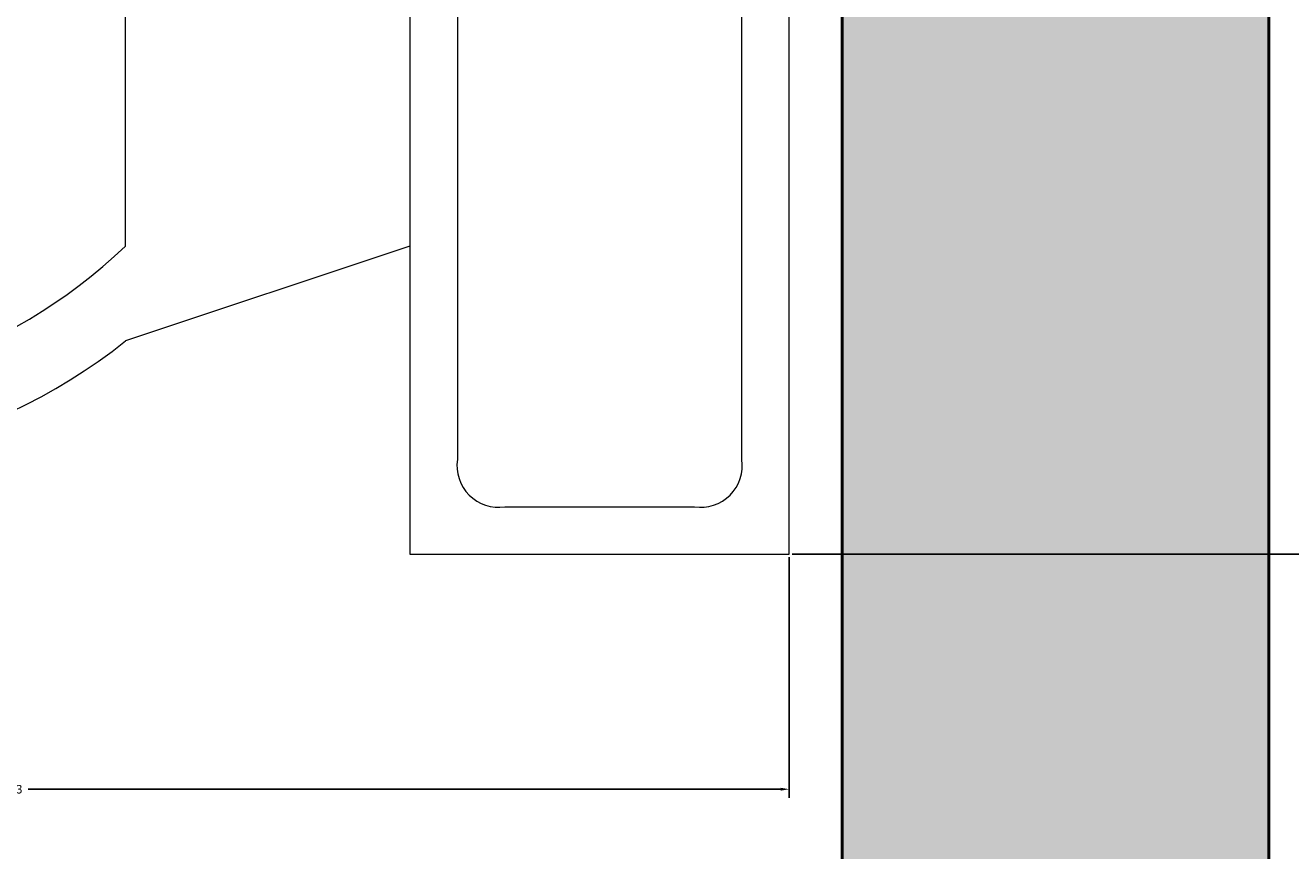
# Model space of a CAD drawing. Units: inches. Extents: x 2307 to 2544, y 2171 to 2540.
# Tile 49 of 52: x 2498 to 2525, y 2482 to 2499. Entities that reach past the tile are written whole.
import ezdxf

# ---------------------------------------------------------------- set-up
doc = ezdxf.new("R2010")
doc.units = ezdxf.units.IN
for name, color, linetype, lineweight in [('A-ANNO-DIMS', 2, 'Continuous', 18), ('A-FLOR-FIXT', 9, 'Continuous', 18), ('A-WALL', 7, 'Continuous', 50)]:
    doc.layers.add(name, color=color, linetype=linetype, lineweight=lineweight)
doc.layers.add('A-WALL-PATT', color=18, linetype='Continuous', lineweight=13, true_color=0x000000)
doc.styles.get("Standard").update_dxf_attribs({"font": 'arial.ttf'})
doc.dimstyles.get("Standard").update_dxf_attribs({"dimtxt": 0.18, "dimasz": 0.18, "dimexe": 0.18, "dimexo": 0.0625, "dimgap": 0.09, "dimtad": 0, "dimtih": 1, "dimtoh": 1, "dimdec": 4, "dimzin": 0, "dimdsep": 46, "dimtxsty": 'Standard', "dimcen": 0.09, "dimadec": 0, "dimazin": 0, "dimtfac": 1, "dimtdec": 4, "dimtofl": 0, "dimtmove": 0, "dimatfit": 3, "dimfxl": 1, "dimtolj": 1, "dimtzin": 0, "dimarcsym": 0})

# ---------------------------------------------------------------- blocks, each defined once
blk = doc.blocks.new('Toilet - top')
for p, q in [((9.5, -6), (9.5, -2)), ((4, -8), (6, -14)), ((4, -14), (-4, -14))]:
    blk.add_line(p, q)
blk.add_lwpolyline([(10.5, -8), (10.5, 0), (-10.5, 0), (-10.5, -8)], close=True)
for points in [[(8.5, -1), (-8.5, -1)], [(-8.5, -7), (8.5, -7)]]:
    blk.add_lwpolyline(points)
for centre, radius, start, end in [((8.625, -1.875), 0.884, 351.8699, 98.1301), ((8.625, -6.125), 0.884, 261.8699, 8.1301), ((-3.519, -21.58), 12.169, 292.0284, 38.5307), ((-4.2, -21.817), 11.329, 301.053, 43.6321)]:
    blk.add_arc(centre, radius, start, end)
blk = doc.blocks.new('*D20')
at = {"layer": 'A-ANNO-DIMS', "color": 0, "lineweight": -2, "transparency": 16777216}
for p, q in [((2481.532, 2488.115), (2481.532, 2483.04)), ((2514.578, 2488.115), (2514.578, 2483.04)), ((2481.712, 2483.22), (2497.588, 2483.22)), ((2514.398, 2483.22), (2498.522, 2483.22))]:
    blk.add_line(p, q, dxfattribs=at)
at = {"layer": 'A-ANNO-DIMS', "color": 0, "transparency": 16777216}
for points in [[(2481.712, 2483.25), (2481.712, 2483.19), (2481.532, 2483.22)], [(2514.398, 2483.25), (2514.398, 2483.19), (2514.578, 2483.22)]]:
    blk.add_solid(points, dxfattribs=at)
at = {"layer": 'Defpoints', "color": 0, "transparency": 16777216}
for p in [(2481.532, 2488.177), (2514.578, 2488.177), (2514.578, 2483.22)]:
    blk.add_point(p, dxfattribs=at)
at = {"layer": 'A-ANNO-DIMS', "color": 0, "transparency": 16777216, "insert": (2498.055, 2483.22), "char_height": 0.18, "attachment_point": 5}
blk.add_mtext('\\A1;WC 33', dxfattribs=at)
blk = doc.blocks.new('*D37')
at = {"layer": 'A-ANNO-DIMS', "color": 0, "lineweight": -2, "transparency": 16777216}
for p, q in [((2524.758, 2520.51), (2544.026, 2520.51)), ((2543.846, 2520.33), (2543.846, 2355.692)), ((2543.846, 2190.69), (2543.846, 2355.328)), ((2524.758, 2190.51), (2544.026, 2190.51))]:
    blk.add_line(p, q, dxfattribs=at)
at = {"layer": 'A-ANNO-DIMS', "color": 0, "transparency": 16777216}
for points in [[(2543.816, 2520.33), (2543.876, 2520.33), (2543.846, 2520.51)], [(2543.816, 2190.69), (2543.876, 2190.69), (2543.846, 2190.51)]]:
    blk.add_solid(points, dxfattribs=at)
at = {"layer": 'Defpoints', "color": 0, "transparency": 16777216}
for p in [(2524.696, 2520.51), (2543.846, 2520.51), (2524.696, 2190.51)]:
    blk.add_point(p, dxfattribs=at)
at = {"layer": 'A-ANNO-DIMS', "color": 0, "transparency": 16777216, "insert": (2543.846, 2355.51), "char_height": 0.18, "attachment_point": 5}
blk.add_mtext('\\A1;330', dxfattribs=at)
blk = doc.blocks.new('*D61')
at = {"layer": 'A-ANNO-DIMS', "color": 0, "lineweight": -2, "transparency": 16777216}
for p, q in [((2491.696, 2435.572), (2491.696, 2540.345)), ((2515.696, 2435.572), (2515.696, 2540.345)), ((2491.876, 2540.165), (2503.476, 2540.165)), ((2515.516, 2540.165), (2503.916, 2540.165))]:
    blk.add_line(p, q, dxfattribs=at)
at = {"layer": 'A-ANNO-DIMS', "color": 0, "transparency": 16777216}
for points in [[(2491.876, 2540.195), (2491.876, 2540.135), (2491.696, 2540.165)], [(2515.516, 2540.195), (2515.516, 2540.135), (2515.696, 2540.165)]]:
    blk.add_solid(points, dxfattribs=at)
at = {"layer": 'Defpoints', "color": 0, "transparency": 16777216}
for p in [(2515.696, 2540.165), (2491.696, 2435.51), (2515.696, 2435.51)]:
    blk.add_point(p, dxfattribs=at)
at = {"layer": 'A-ANNO-DIMS', "color": 0, "transparency": 16777216, "insert": (2503.696, 2540.165), "char_height": 0.18, "attachment_point": 5}
blk.add_mtext('\\A1;24', dxfattribs=at)
blk = doc.blocks.new('*D64')
at = {"layer": 'A-ANNO-DIMS', "color": 0, "lineweight": -2, "transparency": 16777216}
for p, q in [((2515.758, 2511.51), (2544.026, 2511.51)), ((2543.846, 2511.33), (2543.846, 2500.025)), ((2543.846, 2488.357), (2543.846, 2499.661)), ((2514.64, 2488.177), (2544.026, 2488.177))]:
    blk.add_line(p, q, dxfattribs=at)
at = {"layer": 'A-ANNO-DIMS', "color": 0, "transparency": 16777216}
for points in [[(2543.816, 2511.33), (2543.876, 2511.33), (2543.846, 2511.51)], [(2543.816, 2488.357), (2543.876, 2488.357), (2543.846, 2488.177)]]:
    blk.add_solid(points, dxfattribs=at)
at = {"layer": 'Defpoints', "color": 0, "transparency": 16777216}
for p in [(2515.696, 2511.51), (2514.578, 2488.177), (2543.846, 2488.177)]:
    blk.add_point(p, dxfattribs=at)
at = {"layer": 'A-ANNO-DIMS', "color": 0, "transparency": 16777216, "insert": (2543.846, 2499.843), "char_height": 0.18, "attachment_point": 5}
blk.add_mtext('\\A1;23.332', dxfattribs=at)

msp = doc.modelspace()

# ---------------------------------------------------------------- hatches: boundary and pattern name
at = {"layer": 'A-WALL-PATT'}
h = msp.add_hatch(color=256, dxfattribs=at)
h.dxf.hatch_style = 1
h.paths.add_polyline_path([(2433.6935, 2199.5096), (2415.6423, 2199.5096), (2415.6423, 2190.5096), (2433.7832, 2190.5096)], flags=17)
h.paths.add_polyline_path([(2367.6423, 2199.5096), (2335.6958, 2199.5096), (2335.6958, 2307.3983), (2326.6958, 2307.3983), (2326.6958, 2190.5096), (2367.6423, 2190.5096)])
h.paths.add_polyline_path([(2524.6958, 2520.5096), (2496.7832, 2520.5096), (2496.7832, 2515.5149), (2472.7832, 2515.5149), (2472.7832, 2520.5096), (2415.4028, 2520.5096), (2415.4028, 2511.5096), (2451.6958, 2511.5096), (2451.6958, 2439.5096), (2451.6958, 2391.5096), (2445.6958, 2391.5096), (2445.6958, 2387.5096), (2455.6958, 2387.5096), (2455.6958, 2435.5096), (2461.6958, 2435.5096), (2461.6958, 2439.5096), (2455.6958, 2439.5096), (2455.6958, 2511.5096), (2515.6958, 2511.5096), (2515.6958, 2439.5096), (2491.6958, 2439.5096), (2491.6958, 2435.5096), (2515.6958, 2435.5096), (2515.6958, 2319.5096), (2451.6958, 2319.5096), (2451.6958, 2281.5096), (2481.6958, 2281.5096), (2481.6958, 2225.5096), (2485.6958, 2225.5096), (2485.6958, 2285.5096), (2455.6958, 2285.5096), (2455.6958, 2315.5096), (2515.6958, 2315.5096), (2515.6958, 2199.5096), (2469.6952, 2199.5096), (2469.785, 2190.5096), (2524.6958, 2190.5096)])

# ---------------------------------------------------------------- linework, layer by layer
at = {"layer": 'A-WALL'}
msp.add_line((2515.6958, 2511.5096), (2515.6958, 2439.5096), dxfattribs=at)
msp.add_lwpolyline([(2433.7832, 2190.5096), (2326.6958, 2190.5096), (2326.6958, 2520.5096), (2524.6958, 2520.5096), (2524.6958, 2190.5096), (2469.785, 2190.5096)], dxfattribs=at)

# ---------------------------------------------------------------- block references
at = {"layer": 'A-FLOR-FIXT', "rotation": 270}
msp.add_blockref('Toilet - top', (2514.5778, 2498.6772), dxfattribs=at)

# ---------------------------------------------------------------- dimensions: what is measured, and where the dimension line sits
at = {"layer": 'A-ANNO-DIMS'}
dim = msp.add_linear_dim(base=(2515.6958, 2540.1649), p1=(2491.6958, 2435.5096), p2=(2515.6958, 2435.5096), dimstyle='Standard', override={"dimdec": 0, "dimlfac": 1, "dimrnd": 0, "dimzin": 0, "dimdsep": 46, "dimlunit": 2}, dxfattribs=at)
dim.commit()
dim.dimension.update_dxf_attribs({"geometry": '*D61', "text_midpoint": (2503.6958, 2540.1649)})
for base, p1, p2, override, picture, middle in [((2543.8458, 2520.5096), (2524.6958, 2190.5096), (2524.6958, 2520.5096), {"dimdec": 0, "dimlfac": 1, "dimrnd": 0, "dimzin": 0, "dimdsep": 46, "dimlunit": 2}, '*D37', (2543.8458, 2355.5096)), ((2543.8458, 2488.1772), (2515.6958, 2511.5096), (2514.5778, 2488.1772), {"dimdec": 3, "dimlfac": 1, "dimrnd": 0, "dimzin": 0, "dimdsep": 46, "dimlunit": 2}, '*D64', (2543.8458, 2499.8434))]:
    dim = msp.add_linear_dim(base=base, p1=p1, p2=p2, angle=90, dimstyle='Standard', override=override, dxfattribs=at)
    dim.commit()
    dim.dimension.update_dxf_attribs({"geometry": picture, "text_midpoint": middle})
dim = msp.add_linear_dim(base=(2514.5778, 2483.2202), p1=(2481.5315, 2488.1772), p2=(2514.5778, 2488.1772), text='WC <>', dimstyle='Standard', override={"dimdec": 0, "dimlfac": 1, "dimrnd": 0, "dimzin": 0, "dimdsep": 46, "dimlunit": 2}, dxfattribs=at)
dim.commit()
dim.dimension.update_dxf_attribs({"geometry": '*D20', "text_midpoint": (2498.0546, 2483.2202)})

doc.saveas('drawing.dxf')
